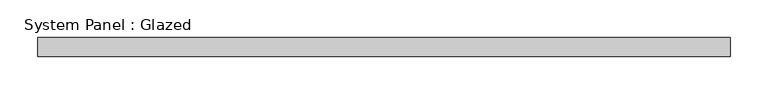
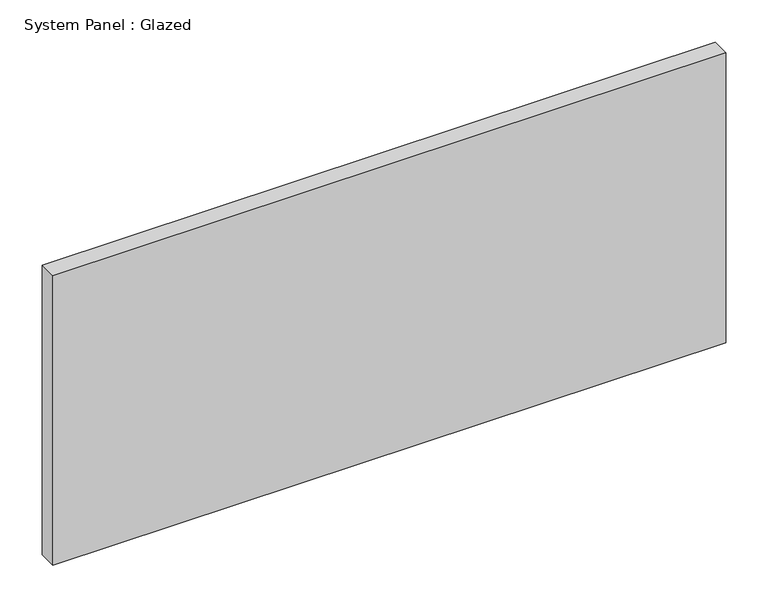
"""IFC4 building model written with IfcOpenShell, lengths in millimetres: plate geometry, System Panel : Glazed."""

from ifc_helpers import new_model, si_unit, origin, origin_with_axes, place, context, project, spatial, polyline, outline, extrude, source, transform, mapped, element, save


def system_panel_glazed_08f033f8(model_context):
    return source(origin(), model_context, "Body", "SweptSolid", [
        extrude(outline(polyline([(460.375, 19.05), (-460.375, 19.05), (-460.375, 44.45), (460.375, 44.45), (460.375, 19.05)])), origin_with_axes(), (0.0, 0.0, 1.0), 419.1),
    ])


if __name__ == "__main__":
    model = new_model("IFC4")
    model_context = context("Model", 3, world=origin())
    ifc_project = project(units=[si_unit("LENGTHUNIT", "METRE", prefix="MILLI")], contexts=[model_context])
    site = spatial("IfcSite", under=ifc_project)
    building = spatial("IfcBuilding", under=site)
    placement = place(None, origin())
    system_panel_glazed_shape = system_panel_glazed_08f033f8(model_context)
    element("IfcPlate", 1, ObjectType="System Panel : Glazed", at=placement, inside=building, context=model_context, shape_type="MappedRepresentation", body=[
        mapped(system_panel_glazed_shape, transform((0.0, 0.0, 0.0), x_axis=(1.0, 0.0, 0.0), y_axis=(0.0, 1.0, 0.0), z_axis=(0.0, 0.0, 1.0))),
    ])
    save(model, "model.ifc")

# Revit data of these elements
# Type "System Panel : Glazed"
#   Construction Type Id = "GSP4R"
#   Analytic Construction = "1/8 in Pilkington single glazing"
#   Visual Light Transmittance = 0.9
#   Solar Heat Gain Coefficient = 0.86
#   Heat Transfer Coefficient (U) = 1.18115 BTU/(h·ft²·°F)
#   Define Thermal Properties by = 1
# Element 1 (IfcPlate, "System Panel : Glazed")
#   Materials on its faces: "Glass"
# Materials
#   "Glass": class "Glass", colour RGB 0 128 192, transparency 0.75, Description = "Soda Lime Glass", Cost = 0
